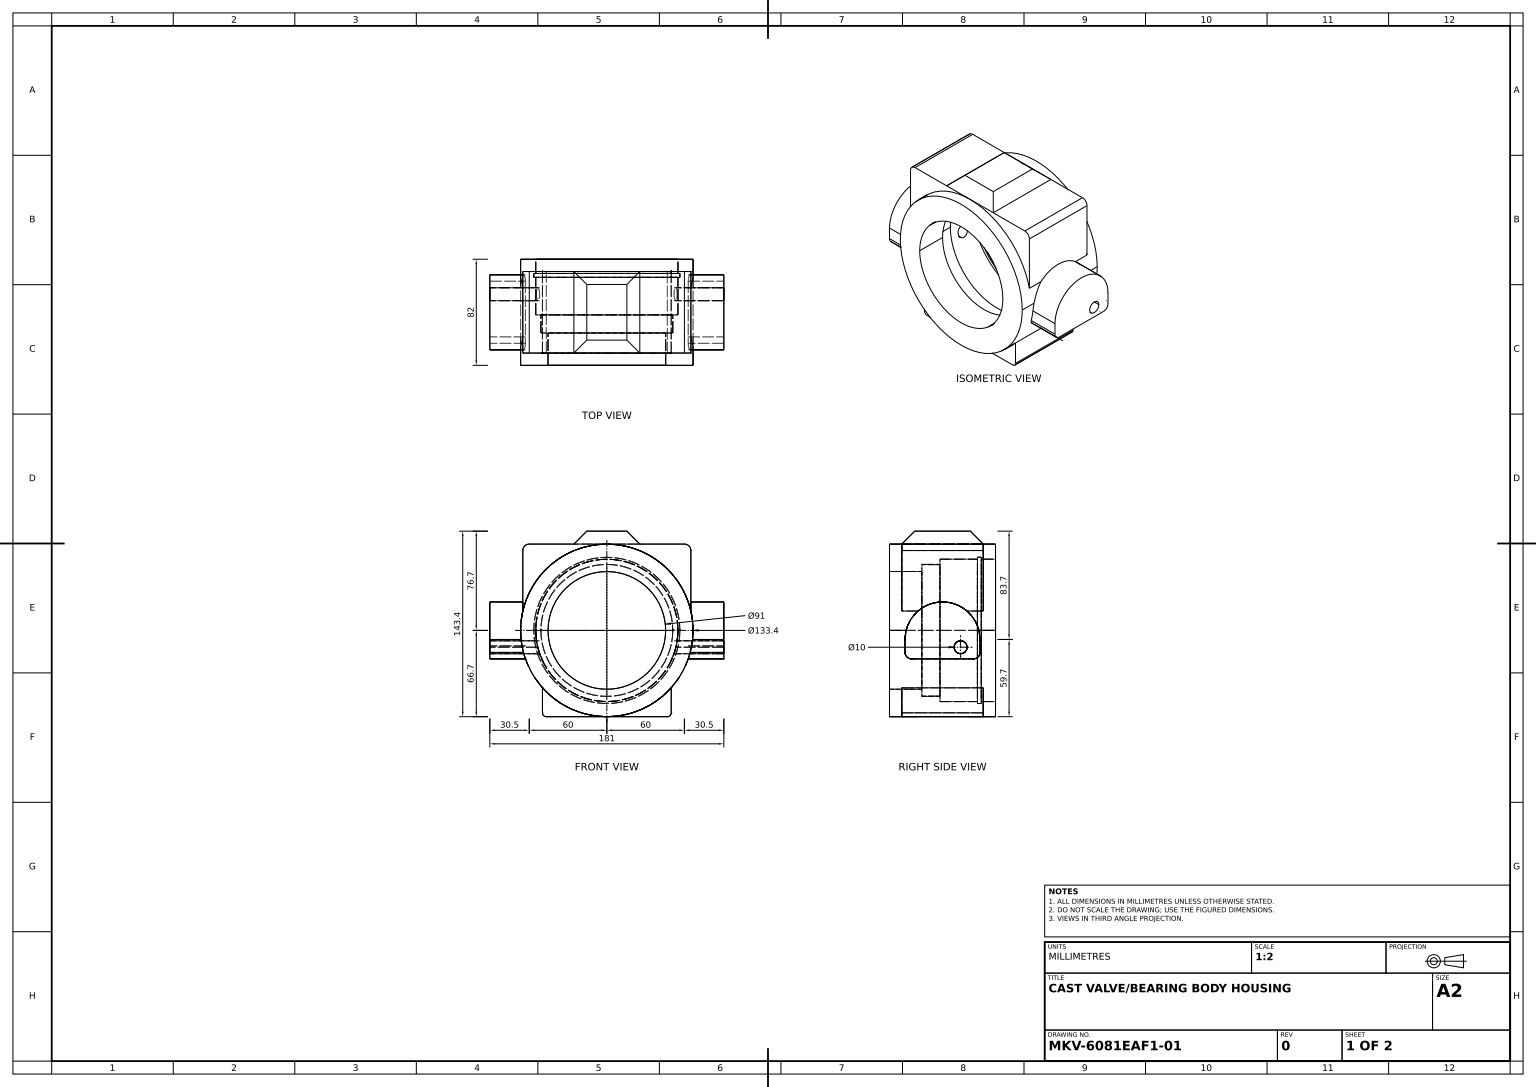
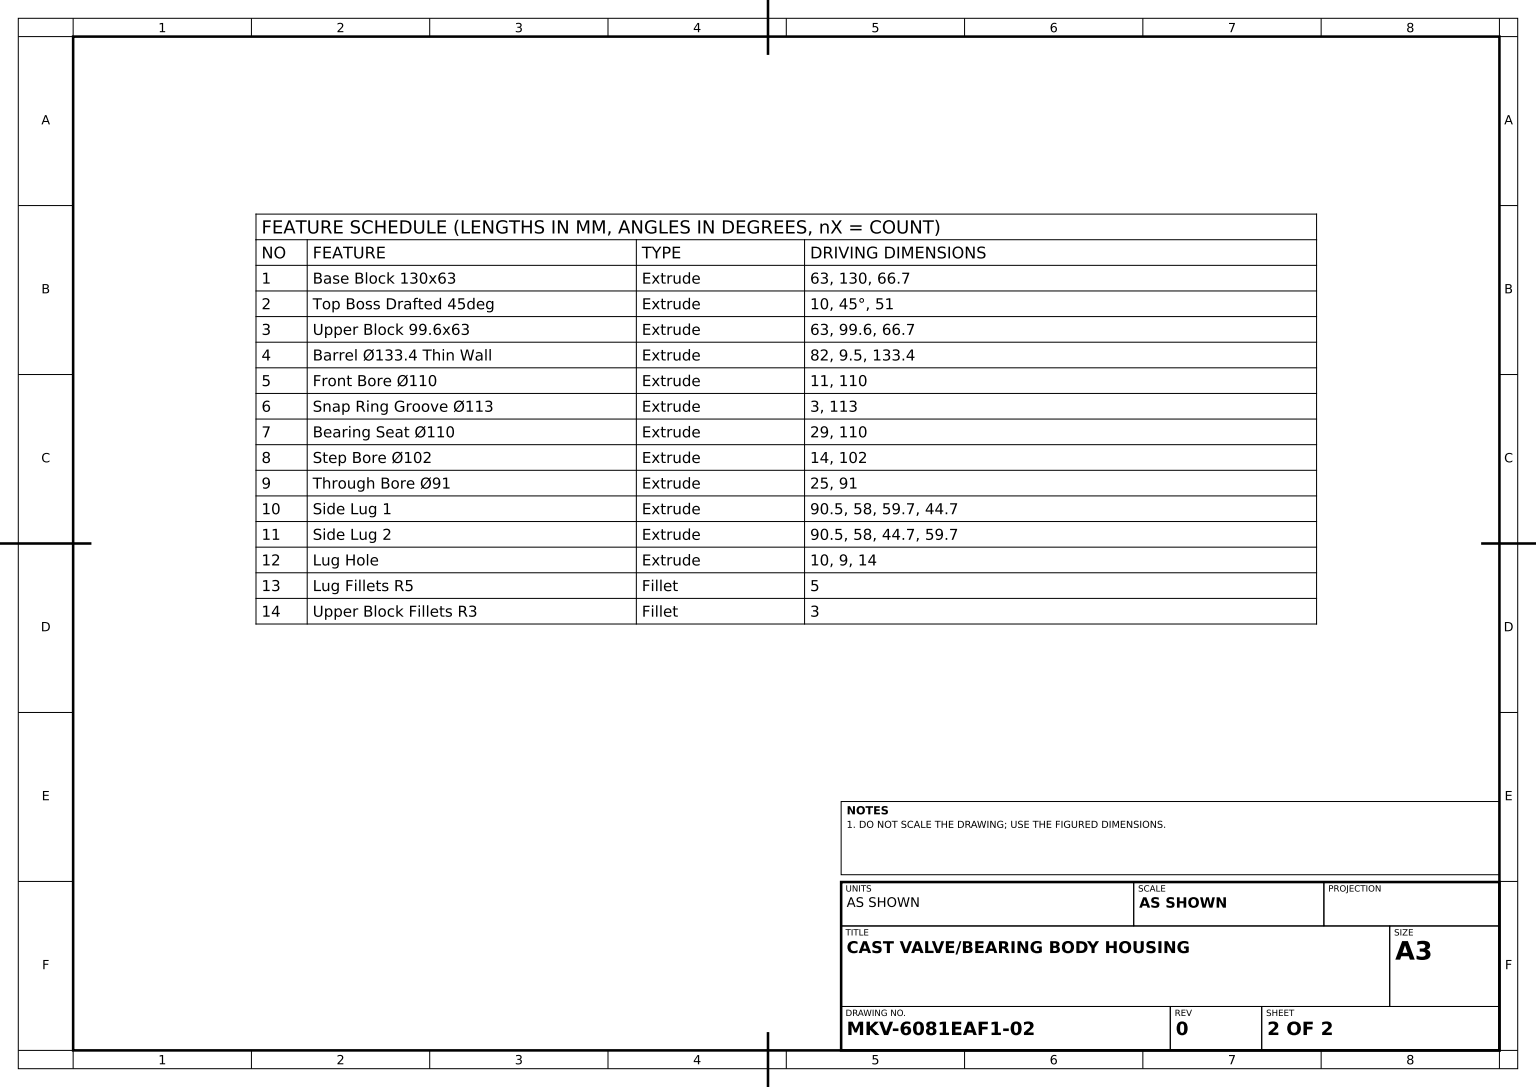
SolidWorks part; units mm, degrees
material "Plain Carbon Steel"
ref_plane "Front Plane" through (0, 0, 0) normal (0, 0, 1) x (1, 0, 0)
ref_plane "Top Plane" through (0, 0, 0) normal (0, 1, 0) x (1, 0, 0)
ref_plane "Right Plane" through (0, 0, 0) normal (1, 0, 0) x (0, 0, -1)
sketch "Base Block Sketch" plane through (0, 0, 0) normal (0, 0, 1) x (1, 0, 0)
  line L1 (-65, -33.35) -> (65, -33.35)
  line L2 (-65, -33.35) -> (-65, 33.35)
  line L3 (-65, 33.35) -> (65, 33.35)
  line L4 (65, -33.35) -> (65, 33.35)
  line L5 (-65, -33.35) -> (65, 33.35) construction
  line L6 (-65, 33.35) -> (65, -33.35) construction
  point P0 (0, 0)
  dimension "D1" = 130
  dimension "D2" = 66.7
extrude "Base Block 130x63" add sketch "Base Block Sketch" along normal mid plane 63
sketch "Top Boss Sketch" plane through (0, 33.35, 0) normal (0, 1, 0) x (1, 0, 0)
  line L0 (65, 31.5) -> (-65, 31.5) construction
  line L1 (-25.5, -31.5) -> (25.5, -31.5)
  line L2 (-25.5, -31.5) -> (-25.5, 31.5)
  line L3 (-25.5, 31.5) -> (25.5, 31.5)
  line L4 (25.5, -31.5) -> (25.5, 31.5)
  line L5 (-25.5, -31.5) -> (25.5, 31.5) construction
  line L6 (-25.5, 31.5) -> (25.5, -31.5) construction
  point P0 (0, 0)
  dimension "D1" = 51
extrude "Top Boss Drafted 45deg" add sketch "Top Boss Sketch" along normal blind 10 draft 45
sketch "Upper Block Sketch" plane through (0, 0, 0) normal (0, 0, 1) x (1, 0, 0)
  line L0 (-65, -33.35) -> (65, -33.35) construction
  line L1 (-49.8, -33.35) -> (49.8, -33.35)
  line L2 (-49.8, -33.35) -> (-49.8, -100.05)
  line L3 (-49.8, -100.05) -> (49.8, -100.05)
  line L4 (49.8, -33.35) -> (49.8, -100.05)
  line L5 (0, 0) -> (0, -12.0065) construction
  dimension "D1" = 99.6
  dimension "D2" = 66.7
extrude "Upper Block 99.6x63" add sketch "Upper Block Sketch" along normal mid plane 63
sketch "Barrel Sketch Ø133.4" plane through (0, 0, 31.5) normal (0, 0, 1) x (1, 0, 0)
  circle A0 centre (0, -33.35) radius 66.7
  dimension "D1" = 133.4
extrude "Barrel Ø133.4 Thin Wall" add sketch "Barrel Sketch Ø133.4" against normal blind 82 from offset 9.5
ref_plane "Lug 1 Plane" through (90.5, 0, 0) normal (1, 0, 0) x (0, 0, -1)
sketch "Side Lug 1 Sketch" plane through (90.5, 0, 0) normal (1, 0, 0) x (0, 0, -1)
  line L0 (-31.5, -100.05) -> (31.5, -100.05) construction
  line L1 (-29, -40.35) -> (-29, -55.35)
  line L2 (-29, -55.35) -> (29, -55.35)
  line L3 (29, -55.35) -> (29, -40.35)
  arc A0 (29, -40.35) -> (-29, -40.35) centre (0, -40.35) ccw
  dimension "D1" = 58
  dimension "D2" = 59.7
  dimension "D3" = 44.7
ref_plane "Lug 2 Plane" through (-90.5, 0, 0) normal (1, 0, 0) x (0, 0, -1)
sketch "Front Bore Sketch Ø110" plane through (0, 0, -41) normal (0, 0, -1) x (-1, 0, 0)
  circle A0 centre (0, -33.35) radius 55
  dimension "D1" = 110
extrude "Front Bore Ø110" cut sketch "Front Bore Sketch Ø110" against normal blind 11
sketch "Snap Ring Groove Sketch Ø113" plane through (0, 0, -30) normal (0, 0, -1) x (-1, 0, 0)
  circle A0 centre (0, -33.35) radius 56.5
  dimension "D1" = 113
extrude "Snap Ring Groove Ø113" cut sketch "Snap Ring Groove Sketch Ø113" against normal blind 3
sketch "Bearing Seat Sketch Ø110" plane through (0, 0, -27) normal (0, 0, -1) x (-1, 0, 0)
  circle A0 centre (0, -33.35) radius 55
  dimension "D1" = 110
extrude "Bearing Seat Ø110" cut sketch "Bearing Seat Sketch Ø110" against normal blind 29
sketch "Step Bore Sketch Ø102" plane through (0, 0, 2) normal (0, 0, -1) x (-1, 0, 0)
  circle A0 centre (0, -33.35) radius 51
  dimension "D1" = 102
extrude "Step Bore Ø102" cut sketch "Step Bore Sketch Ø102" against normal blind 14
sketch "Through Bore Sketch Ø91" plane through (0, 0, 16) normal (0, 0, -1) x (-1, 0, 0)
  circle A0 centre (0, -33.35) radius 45.5
  dimension "D1" = 91
extrude "Through Bore Ø91" cut sketch "Through Bore Sketch Ø91" against normal blind 25
extrude "Side Lug 1" add sketch "Side Lug 1 Sketch" against normal up to next
sketch "Side Lug 2 Sketch" plane through (-90.5, 0, 0) normal (1, 0, 0) x (0, 0, -1)
  line L0 (29, -55.35) -> (-29, -55.35)
  line L1 (29, -40.35) -> (29, -55.35)
  line L2 (-29, -55.35) -> (-29, -40.35)
  line L3 (-31.5, -100.05) -> (31.5, -100.05) construction
  arc A0 (29, -40.35) -> (-29, -40.35) centre (0, -40.35) ccw
  dimension "D1" = 58
  dimension "D2" = 44.7
  dimension "D3" = 59.7
extrude "Side Lug 2" add sketch "Side Lug 2 Sketch" along normal up to next
sketch "Lug Hole Sketch" plane through (-90.5, 0, 0) normal (-1, 0, 0) x (0, 0, 1)
  line L0 (-29, -55.35) -> (29, -55.35) construction
  circle A0 centre (-14, -46.35) radius 5
  dimension "D1" = 10
  dimension "D2" = 9
  dimension "D3" = 14
extrude "Lug Hole" cut sketch "Lug Hole Sketch" against normal through all
fillet "Lug Fillets R5" radius 5 6 edges at (65, 33.35, 0) (-65, 33.35, 0) (76.7337, -55.35, 29) (76.7337, -55.35, -29) (-76.7337, -55.35, 29) (-76.7337, -55.35, -29)
fillet "Upper Block Fillets R3" radius 3 2 edges at (49.8, -100.05, 0) (-49.8, -100.05, 0)
